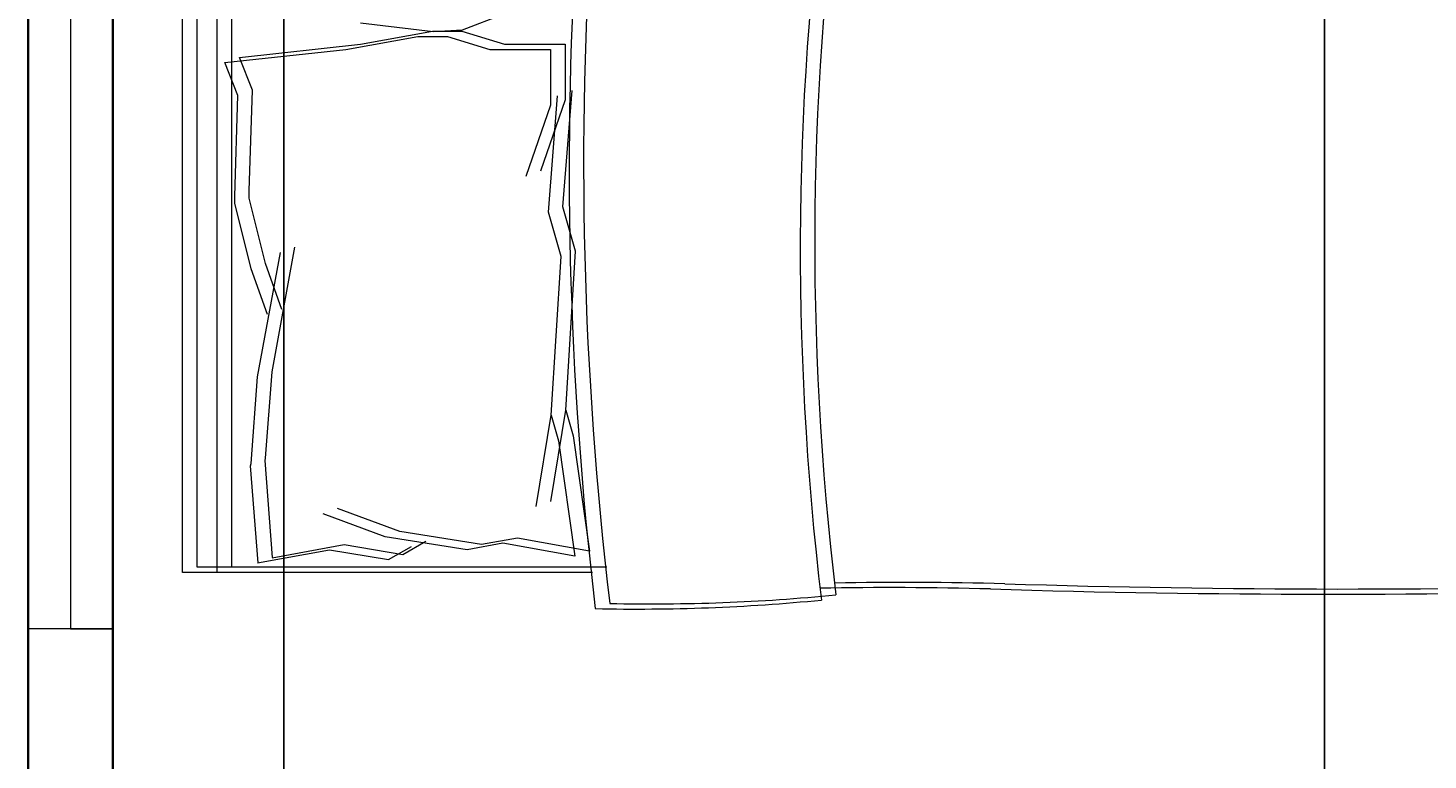
# Model space of a CAD drawing. Units: inches. Extents: x 1088 to 1703, y 668 to 1875.
# Tile 15 of 45: x 1170 to 1245, y 1711 to 1750. Entities that reach past the tile are written whole.
import ezdxf

# ---------------------------------------------------------------- set-up
doc = ezdxf.new("R2010")
doc.units = ezdxf.units.IN
for name, color, linetype, lineweight in [('A-ANNO-DIMS', 2, 'Continuous', 18), ('A-FURN', 8, 'Continuous', 13), ('A-GLAZ', 4, 'Continuous', 18), ('A-WALL', 7, 'Continuous', 35)]:
    doc.layers.add(name, color=color, linetype=linetype, lineweight=lineweight)
doc.styles.get("Standard").update_dxf_attribs({"font": 'arial.ttf'})
doc.dimstyles.get("Standard").update_dxf_attribs({"dimtxt": 0.18, "dimasz": 0.18, "dimexe": 0.18, "dimexo": 0.0625, "dimgap": 0.09, "dimtad": 0, "dimtih": 1, "dimtoh": 1, "dimdec": 4, "dimzin": 0, "dimdsep": 46, "dimtxsty": 'Standard', "dimcen": 0.09, "dimadec": 0, "dimazin": 0, "dimtfac": 1, "dimtdec": 4, "dimtofl": 0, "dimtmove": 0, "dimatfit": 3, "dimfxl": 1, "dimtolj": 1, "dimtzin": 0, "dimarcsym": 0})

# ---------------------------------------------------------------- blocks, each defined once
blk = doc.blocks.new('BED-DOUBLE')
for p, q in [((0.766, 4.44), (0.766, 61.734)), ((2.605, 4.44), (2.605, 61.734)), ((0, 4.167), (0, 61.46)), ((1.838, 4.167), (1.838, 61.46)), ((14.838, 32.892), (17.044, 33.725)), ((9.422, 32.117), (13.236, 32.81)), ((9.432, 33.249), (13.281, 32.795)), ((13.236, 32.81), (14.796, 32.81)), ((13.281, 32.795), (14.838, 32.892)), ((14.796, 32.81), (17.049, 32.117)), ((3.008, 31.424), (9.422, 32.117)), ((8.656, 31.843), (12.469, 32.536)), ((12.469, 32.536), (14.029, 32.536)), ((14.029, 32.536), (16.283, 31.843)), ((17.049, 32.117), (20.264, 32.117)), ((20.264, 32.117), (20.264, 29.171)), ((2.242, 31.15), (8.656, 31.843)), ((3.702, 29.691), (3.008, 31.424)), ((16.283, 31.843), (19.497, 31.843)), ((19.497, 31.843), (19.497, 28.897)), ((2.935, 29.417), (2.242, 31.15)), ((3.528, 24.361), (3.702, 29.691)), ((2.762, 24.087), (2.935, 29.417)), ((20.264, 29.171), (18.956, 25.401)), ((19.384, 23.239), (19.868, 29.391)), ((20.151, 23.513), (20.635, 29.665)), ((19.497, 28.897), (18.189, 25.127)), ((2.762, 23.701), (2.762, 24.087)), ((3.528, 23.975), (3.528, 24.361)), ((4.395, 20.509), (3.528, 23.975)), ((3.629, 20.235), (2.762, 23.701)), ((20.052, 20.889), (19.384, 23.239)), ((20.819, 21.163), (20.151, 23.513)), ((3.975, 14.516), (5.189, 21.102)), ((4.742, 14.79), (5.955, 21.376)), ((19.536, 12.485), (20.052, 20.889)), ((20.302, 12.759), (20.819, 21.163)), ((4.495, 17.809), (3.629, 20.235)), ((5.262, 18.083), (4.395, 20.509)), ((3.629, 9.933), (3.975, 14.516)), ((4.395, 10.206), (4.742, 14.79)), ((19.503, 7.925), (20.302, 12.759)), ((20.302, 12.759), (20.689, 11.4)), ((18.736, 7.651), (19.536, 12.485)), ((19.536, 12.485), (19.923, 11.126)), ((19.923, 11.126), (20.789, 5.016)), ((20.689, 11.4), (21.556, 5.29)), ((3.607, 9.806), (3.629, 9.933)), ((4.002, 4.674), (3.607, 9.806)), ((4.373, 10.08), (4.395, 10.206)), ((4.768, 4.948), (4.373, 10.08)), ((11.502, 6.33), (8.209, 7.543)), ((10.736, 6.056), (7.442, 7.269)), ((15.069, 5.363), (10.736, 6.056)), ((15.836, 5.637), (11.502, 6.33)), ((17.742, 5.983), (15.836, 5.637)), ((21.556, 5.29), (17.742, 5.983)), ((3.975, 4.67), (7.789, 5.363)), ((4.742, 4.943), (8.555, 5.637)), ((7.789, 5.363), (10.909, 4.843)), ((8.555, 5.637), (11.675, 5.117)), ((10.909, 4.843), (12.122, 5.536)), ((11.675, 5.117), (12.889, 5.81)), ((16.976, 5.709), (15.069, 5.363)), ((20.789, 5.016), (16.976, 5.709)), ((21.712, 4.167), (0, 4.167)), ((22.478, 4.44), (0.766, 4.44))]:
    blk.add_line(p, q)
for centre, radius, start, end in [((187.401, 21.287), 154.676, 171.78449, 186.90062), ((188.167, 21.561), 154.676, 171.78449, 186.90062), ((219.021, 25.88), 197.774, 176.08655, 186.78213), ((218.255, 25.607), 197.774, 176.08655, 186.78213), ((24.859, 102.371), 99.872, 268.72178, 275.60397), ((37.373, -200.577), 203.938, 88.4762, 91.00819), ((38.139, -200.304), 203.938, 88.4762, 91.00819), ((60.679, 581.233), 578.221, 268.227709, 271.718541), ((61.445, 581.507), 578.221, 268.227709, 271.718541), ((24.093, 102.097), 99.872, 268.72178, 275.60397)]:
    blk.add_arc(centre, radius, start, end)
blk = doc.blocks.new('*D28')
at = {"layer": 'A-ANNO-DIMS', "color": 0, "lineweight": -2, "transparency": 16777216}
for p, q in [((1170.345, 1803.621), (1170.345, 1857.788)), ((1170.525, 1857.608), (1408.147, 1857.608)), ((1646.563, 1857.608), (1408.941, 1857.608)), ((1646.743, 1745.552), (1646.743, 1857.788))]:
    blk.add_line(p, q, dxfattribs=at)
at = {"layer": 'A-ANNO-DIMS', "color": 0, "transparency": 16777216}
for points in [[(1170.525, 1857.638), (1170.525, 1857.578), (1170.345, 1857.608)], [(1646.563, 1857.638), (1646.563, 1857.578), (1646.743, 1857.608)]]:
    blk.add_solid(points, dxfattribs=at)
at = {"layer": 'Defpoints', "color": 0, "transparency": 16777216}
for p in [(1646.743, 1857.608), (1170.345, 1803.558), (1646.743, 1745.49)]:
    blk.add_point(p, dxfattribs=at)
at = {"layer": 'A-ANNO-DIMS', "color": 0, "transparency": 16777216, "insert": (1408.544, 1857.608), "char_height": 0.18, "attachment_point": 5}
blk.add_mtext('\\A1;476.4', dxfattribs=at)
blk = doc.blocks.new('*D35')
at = {"layer": 'A-ANNO-DIMS', "color": 0, "lineweight": -2, "transparency": 16777216}
for p, q in [((1183.893, 1448.103), (1183.893, 1857.788)), ((1184.073, 1857.608), (1211.072, 1857.608)), ((1238.859, 1857.608), (1211.86, 1857.608)), ((1239.039, 1448.103), (1239.039, 1857.788))]:
    blk.add_line(p, q, dxfattribs=at)
at = {"layer": 'A-ANNO-DIMS', "color": 0, "transparency": 16777216}
for points in [[(1184.073, 1857.638), (1184.073, 1857.578), (1183.893, 1857.608)], [(1238.859, 1857.638), (1238.859, 1857.578), (1239.039, 1857.608)]]:
    blk.add_solid(points, dxfattribs=at)
at = {"layer": 'Defpoints', "color": 0, "transparency": 16777216}
for p in [(1239.039, 1857.608), (1183.893, 1448.04), (1239.039, 1448.04)]:
    blk.add_point(p, dxfattribs=at)
at = {"layer": 'A-ANNO-DIMS', "color": 0, "transparency": 16777216, "insert": (1211.466, 1857.608), "char_height": 0.18, "attachment_point": 5}
blk.add_mtext('\\A1;55.15', dxfattribs=at)

msp = doc.modelspace()

# ---------------------------------------------------------------- linework, layer by layer
at = {"layer": 'A-GLAZ'}
for p, q in [((1172.595, 1777.837), (1172.595, 1717.837)), ((1174.845, 1717.837), (1170.345, 1717.837)), ((1172.595, 1717.837), (1174.845, 1717.837))]:
    msp.add_line(p, q, dxfattribs=at)
at = {"layer": 'A-WALL'}
for p, q in [((1170.345, 1803.558), (1170.345, 836.058)), ((1174.845, 1799.058), (1174.845, 1649.058))]:
    msp.add_line(p, q, dxfattribs=at)

# ---------------------------------------------------------------- block references
at = {"layer": 'A-FURN'}
msp.add_blockref('BED-DOUBLE', (1178.533, 1716.657), dxfattribs=at)

# ---------------------------------------------------------------- dimensions: what is measured, and where the dimension line sits
at = {"layer": 'A-ANNO-DIMS'}
for base, p1, p2, override, picture, middle in [((1646.743, 1857.608), (1170.345, 1803.558), (1646.743, 1745.49), {"dimdec": 1, "dimlfac": 1, "dimrnd": 0, "dimzin": 0, "dimdsep": 46, "dimlunit": 2}, '*D28', (1408.544, 1857.608)), ((1239.039, 1857.608), (1183.893, 1448.04), (1239.039, 1448.04), {"dimdec": 2, "dimlfac": 1, "dimrnd": 0, "dimzin": 0, "dimdsep": 46, "dimlunit": 2}, '*D35', (1211.466, 1857.608))]:
    dim = msp.add_linear_dim(base=base, p1=p1, p2=p2, dimstyle='Standard', override=override, dxfattribs=at)
    dim.commit()
    dim.dimension.update_dxf_attribs({"geometry": picture, "text_midpoint": middle})

doc.saveas('drawing.dxf')
